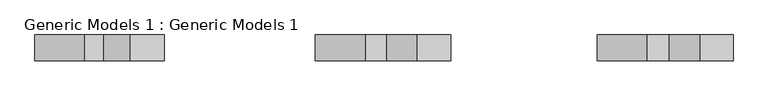
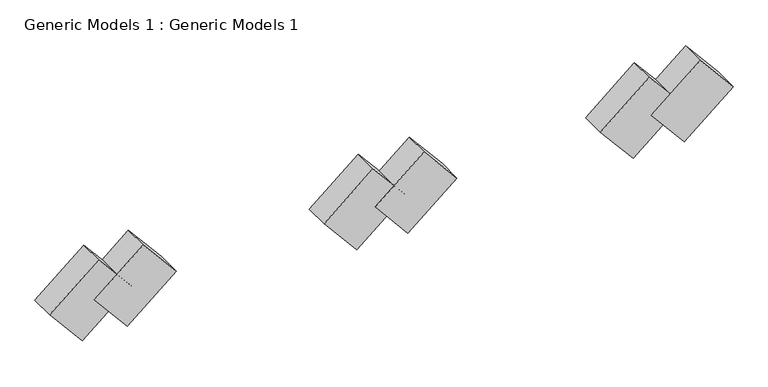
"""IFC4 building model written with IfcOpenShell, lengths in millimetres: proxy geometry, Generic Models 1 : Generic Models 1."""

from ifc_helpers import new_model, si_unit, frame, origin, place, context, project, spatial, polyline, outline, extrude, source, transform, mapped, element, save


def generic_models_1_generic_models_1_8d9aa75c(model_context):
    return source(origin(), model_context, "Body", "SweptSolid", [
        extrude(outline(polyline([(0.0, -761.9999999), (0.0, 0.0), (304.8, 0.0), (304.8, -761.9999999), (0.0, -761.9999999)])), frame((7719.7433269, 2597.6372886, 202.1212911), z_axis=(-0.6427876096865395, 0.0, 0.7660444431189779), x_axis=(0.0, 1.0, 0.0)), (0.0, 0.0, 1.0), 609.6),
        extrude(outline(polyline([(0.0, -761.9999999), (0.0, 0.0), (304.8, 0.0), (304.8, -761.9999999), (0.0, -761.9999999)])), frame((7110.1433269, 2597.6372886, 202.1212911), z_axis=(-0.6427876096865395, 0.0, 0.766044443118978), x_axis=(0.0, 1.0, 0.0)), (0.0, 0.0, 1.0), 609.6),
        extrude(outline(polyline([(0.0, -761.9999999), (0.0, 0.0), (304.8, 0.0), (304.8, -761.9999999), (0.0, -761.9999999)])), frame((4421.2932471, 2597.6372886, 202.1212911), z_axis=(-0.6427876096865383, 0.0, 0.766044443118979), x_axis=(0.0, 1.0, 0.0)), (0.0, 0.0, 1.0), 609.6),
        extrude(outline(polyline([(0.0, -761.9999999), (0.0, 0.0), (304.8, 0.0), (304.8, -761.9999999), (0.0, -761.9999999)])), frame((3811.6932471, 2597.6372886, 202.1212911), z_axis=(-0.6427876096865386, 0.0, 0.7660444431189787), x_axis=(0.0, 1.0, 0.0)), (0.0, 0.0, 1.0), 609.6),
        extrude(outline(polyline([(0.0, -761.9999999), (0.0, 0.0), (304.8, 0.0), (304.8, -761.9999999), (0.0, -761.9999999)])), frame((1068.4932471, 2597.6372886, 202.1212911), z_axis=(-0.6427876096865387, 0.0, 0.7660444431189787), x_axis=(0.0, 1.0, 0.0)), (0.0, 0.0, 1.0), 609.6),
        extrude(outline(polyline([(0.0, -761.9999999), (0.0, 0.0), (304.8, 0.0), (304.8, -761.9999999), (0.0, -761.9999999)])), frame((535.0932471, 2597.6372886, 202.1212911), z_axis=(-0.6427876096865386, 0.0, 0.7660444431189788), x_axis=(0.0, 1.0, 0.0)), (0.0, 0.0, 1.0), 609.6),
    ])


if __name__ == "__main__":
    model = new_model("IFC4")
    model_context = context("Model", 3, world=origin())
    ifc_project = project(units=[si_unit("LENGTHUNIT", "METRE", prefix="MILLI")], contexts=[model_context])
    site = spatial("IfcSite", under=ifc_project)
    building = spatial("IfcBuilding", under=site)
    placement = place(None, origin())
    generic_models_1_generic_models_1_shape = generic_models_1_generic_models_1_8d9aa75c(model_context)
    element("IfcBuildingElementProxy", 1, Name="Generic Models 1 : Generic Models 1", ObjectType="Generic Models 1 : Generic Models 1", at=placement, inside=building, context=model_context, shape_type="MappedRepresentation", body=[
        mapped(generic_models_1_generic_models_1_shape, transform((0.0, 0.0, 0.0), x_axis=(1.0, 0.0, 0.0), y_axis=(0.0, 1.0, 0.0), z_axis=(0.0, 0.0, 1.0))),
    ])
    save(model, "model.ifc")

# Revit data of these elements
# Element 1 (IfcBuildingElementProxy, "Generic Models 1 : Generic Models 1")
#   Materials on its faces: "Carpet (1)"
# Materials
#   "Carpet (1)": class "Carpet", colour RGB 124 80 67, transparency 0, Description = "Interior finish", Cost = 0
